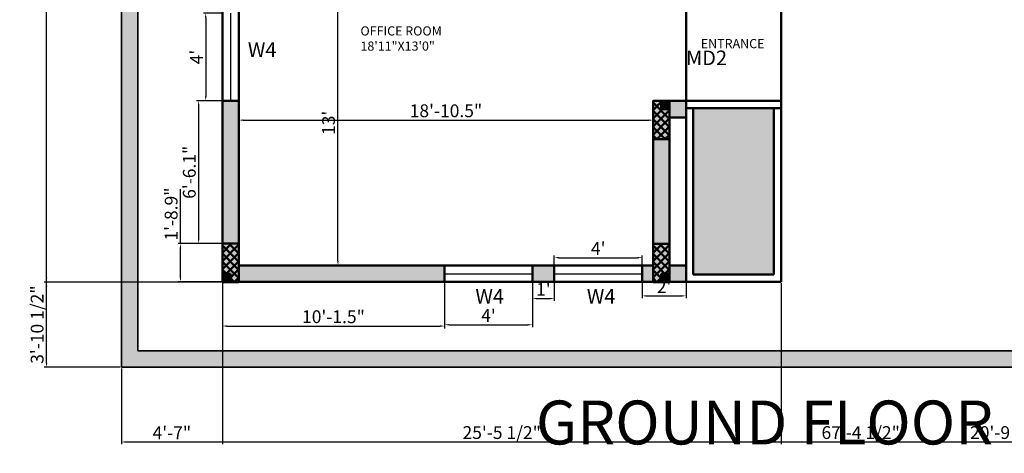
# Model space of a CAD drawing. Units: inches. Extents: x 1749 to 3550, y 1117 to 2383.
# Tile 6 of 15: x 1749 to 2287, y 1756 to 1993. Entities that reach past the tile are written whole.
import ezdxf

# ---------------------------------------------------------------- set-up
doc = ezdxf.new("R2010")
doc.units = ezdxf.units.IN
for name, color, linetype, lineweight in [('A-ANNO-DIMS', 2, 'Continuous', 18), ('A-ANNO-TEXT', 3, 'Continuous', 18), ('A-AREA-IDEN', 7, 'Continuous', 18), ('A-COLS', 10, 'Continuous', 50), ('A-GLAZ', 4, 'Continuous', 25), ('A-WALL', 7, 'Continuous', 50), ('A-WALL-PATT', 8, 'Continuous', 13), ('C-PROP', 8, 'Continuous', 35)]:
    doc.layers.add(name, color=color, linetype=linetype, lineweight=lineweight)
doc.styles.get("Standard").update_dxf_attribs({"font": 'arial.ttf'})
doc.dimstyles.new('ISO-25', dxfattribs={"dimtxt": 7, "dimasz": 2.5, "dimexe": 1.25, "dimexo": 0.625, "dimtad": 1, "dimdec": 1, "dimlunit": 3, "dimtxsty": 'Standard', "dimcen": 2.5, "dimadec": 0, "dimazin": 0, "dimtfac": 1, "dimtdec": 1, "dimtmove": 0, "dimatfit": 3, "dimfxl": 1, "dimarcsym": 0})

# ---------------------------------------------------------------- blocks, each defined once
blk = doc.blocks.new('*D6')
at = {"layer": 'A-ANNO-DIMS', "color": 0, "lineweight": -2, "transparency": 16777216}
for p, q in [((1923.39, 2014.66), (1924.02, 2014.66)), ((1922.77, 1861.16), (1922.77, 2012.16)), ((1923.39, 1858.66), (1924.02, 1858.66))]:
    blk.add_line(p, q, dxfattribs=at)
at = {"layer": 'A-ANNO-DIMS', "color": 0, "transparency": 16777216}
for points in [[(1922.35, 2012.16), (1923.18, 2012.16), (1922.77, 2014.66)], [(1922.35, 1861.16), (1923.18, 1861.16), (1922.77, 1858.66)]]:
    blk.add_solid(points, dxfattribs=at)
at = {"layer": 'Defpoints', "color": 0, "transparency": 16777216}
for p in [(1922.77, 2014.66), (1922.77, 2014.66), (1922.77, 1858.66)]:
    blk.add_point(p, dxfattribs=at)
at = {"layer": 'A-ANNO-DIMS', "color": 0, "transparency": 16777216, "insert": (1918.57, 1936.66), "char_height": 7, "attachment_point": 5, "rotation": 90}
blk.add_mtext("13'", dxfattribs=at)
blk = doc.blocks.new('*D7')
at = {"layer": 'A-ANNO-DIMS', "color": 0, "lineweight": -2, "transparency": 16777216}
for p, q in [((1868.6, 1948.04), (1868.6, 1936.91)), ((2095.1, 1948.04), (2095.1, 1936.91)), ((1871.1, 1938.16), (2092.6, 1938.16))]:
    blk.add_line(p, q, dxfattribs=at)
at = {"layer": 'A-ANNO-DIMS', "color": 0, "transparency": 16777216}
for points in [[(1871.1, 1938.58), (1871.1, 1937.74), (1868.6, 1938.16)], [(2092.6, 1938.58), (2092.6, 1937.74), (2095.1, 1938.16)]]:
    blk.add_solid(points, dxfattribs=at)
at = {"layer": 'Defpoints', "color": 0, "transparency": 16777216}
for p in [(1868.6, 1948.66), (2095.1, 1948.66), (2095.1, 1938.16)]:
    blk.add_point(p, dxfattribs=at)
at = {"layer": 'A-ANNO-DIMS', "color": 0, "transparency": 16777216, "insert": (1981.85, 1942.36), "char_height": 7, "attachment_point": 5}
blk.add_mtext('18\'-10.5"', dxfattribs=at)
blk = doc.blocks.new('*D88')
at = {"layer": 'A-ANNO-DIMS', "color": 0, "lineweight": -2, "ltscale": 0.5, "transparency": 16777216}
for p, q in [((1858.98, 1996.66), (1849.23, 1996.66)), ((1850.48, 1994.16), (1850.48, 1951.16)), ((1858.98, 1948.66), (1849.23, 1948.66))]:
    blk.add_line(p, q, dxfattribs=at)
at = {"layer": 'A-ANNO-DIMS', "color": 0, "ltscale": 0.5, "transparency": 16777216}
for points in [[(1850.06, 1994.16), (1850.89, 1994.16), (1850.48, 1996.66)], [(1850.06, 1951.16), (1850.89, 1951.16), (1850.48, 1948.66)]]:
    blk.add_solid(points, dxfattribs=at)
at = {"layer": 'Defpoints', "color": 0, "ltscale": 0.5, "transparency": 16777216}
for p in [(1859.6, 1996.66), (1850.48, 1948.66), (1859.6, 1948.66)]:
    blk.add_point(p, dxfattribs=at)
at = {"layer": 'A-ANNO-DIMS', "color": 0, "ltscale": 0.5, "transparency": 16777216, "insert": (1846.35, 1972.66), "char_height": 7, "attachment_point": 5, "rotation": 90}
blk.add_mtext("4'", dxfattribs=at)
blk = doc.blocks.new('*D89')
at = {"layer": 'A-ANNO-DIMS', "color": 0, "lineweight": -2, "ltscale": 0.5, "transparency": 16777216}
for p, q in [((1858.98, 1948.66), (1845.38, 1948.66)), ((1846.63, 1946.16), (1846.63, 1873.11)), ((1858.98, 1870.61), (1845.38, 1870.61))]:
    blk.add_line(p, q, dxfattribs=at)
at = {"layer": 'A-ANNO-DIMS', "color": 0, "ltscale": 0.5, "transparency": 16777216}
for points in [[(1846.21, 1946.16), (1847.04, 1946.16), (1846.63, 1948.66)], [(1846.21, 1873.11), (1847.04, 1873.11), (1846.63, 1870.61)]]:
    blk.add_solid(points, dxfattribs=at)
at = {"layer": 'Defpoints', "color": 0, "ltscale": 0.5, "transparency": 16777216}
for p in [(1859.6, 1948.66), (1846.63, 1870.61), (1859.6, 1870.61)]:
    blk.add_point(p, dxfattribs=at)
at = {"layer": 'A-ANNO-DIMS', "color": 0, "ltscale": 0.5, "transparency": 16777216, "insert": (1842.43, 1909.63), "char_height": 7, "attachment_point": 5, "rotation": 90}
blk.add_mtext('6\'-6.1"', dxfattribs=at)
blk = doc.blocks.new('*D90')
at = {"layer": 'A-ANNO-DIMS', "color": 0, "lineweight": -2, "ltscale": 0.5, "transparency": 16777216}
for p, q in [((1836.69, 1870.61), (1836.69, 1900.46)), ((1858.98, 1870.61), (1835.44, 1870.61)), ((1836.69, 1852.16), (1836.69, 1868.11)), ((1858.98, 1849.66), (1835.44, 1849.66))]:
    blk.add_line(p, q, dxfattribs=at)
at = {"layer": 'A-ANNO-DIMS', "color": 0, "ltscale": 0.5, "transparency": 16777216}
for points in [[(1836.28, 1868.11), (1837.11, 1868.11), (1836.69, 1870.61)], [(1836.28, 1852.16), (1837.11, 1852.16), (1836.69, 1849.66)]]:
    blk.add_solid(points, dxfattribs=at)
at = {"layer": 'Defpoints', "color": 0, "ltscale": 0.5, "transparency": 16777216}
for p in [(1836.69, 1870.61), (1859.6, 1870.61), (1859.6, 1849.66)]:
    blk.add_point(p, dxfattribs=at)
at = {"layer": 'A-ANNO-DIMS', "color": 0, "ltscale": 0.5, "transparency": 16777216, "insert": (1832.49, 1886.78), "char_height": 7, "attachment_point": 5, "rotation": 90}
blk.add_mtext('1\'-8.9"', dxfattribs=at)
blk = doc.blocks.new('*D91')
at = {"layer": 'A-ANNO-DIMS', "color": 0, "lineweight": -2, "ltscale": 0.5, "transparency": 16777216}
for p, q in [((1859.6, 1849.04), (1859.6, 1824.26)), ((1981.1, 1849.04), (1981.1, 1824.26)), ((1862.1, 1825.51), (1978.6, 1825.51))]:
    blk.add_line(p, q, dxfattribs=at)
at = {"layer": 'A-ANNO-DIMS', "color": 0, "ltscale": 0.5, "transparency": 16777216}
for points in [[(1862.1, 1825.93), (1862.1, 1825.1), (1859.6, 1825.51)], [(1978.6, 1825.93), (1978.6, 1825.1), (1981.1, 1825.51)]]:
    blk.add_solid(points, dxfattribs=at)
at = {"layer": 'Defpoints', "color": 0, "ltscale": 0.5, "transparency": 16777216}
for p in [(1859.6, 1849.66), (1981.1, 1849.66), (1981.1, 1825.51)]:
    blk.add_point(p, dxfattribs=at)
at = {"layer": 'A-ANNO-DIMS', "color": 0, "ltscale": 0.5, "transparency": 16777216, "insert": (1920.35, 1829.71), "char_height": 7, "attachment_point": 5}
blk.add_mtext('10\'-1.5"', dxfattribs=at)
blk = doc.blocks.new('*D92')
at = {"layer": 'A-ANNO-DIMS', "color": 0, "lineweight": -2, "ltscale": 0.5, "transparency": 16777216}
for p, q in [((1981.1, 1849.04), (1981.1, 1824.98)), ((2029.1, 1849.04), (2029.1, 1824.98)), ((1983.6, 1826.23), (2026.6, 1826.23))]:
    blk.add_line(p, q, dxfattribs=at)
at = {"layer": 'A-ANNO-DIMS', "color": 0, "ltscale": 0.5, "transparency": 16777216}
for points in [[(1983.6, 1826.64), (1983.6, 1825.81), (1981.1, 1826.23)], [(2026.6, 1826.64), (2026.6, 1825.81), (2029.1, 1826.23)]]:
    blk.add_solid(points, dxfattribs=at)
at = {"layer": 'Defpoints', "color": 0, "ltscale": 0.5, "transparency": 16777216}
for p in [(1981.1, 1849.66), (2029.1, 1849.66), (2029.1, 1826.23)]:
    blk.add_point(p, dxfattribs=at)
at = {"layer": 'A-ANNO-DIMS', "color": 0, "ltscale": 0.5, "transparency": 16777216, "insert": (2005.1, 1830.35), "char_height": 7, "attachment_point": 5}
blk.add_mtext("4'", dxfattribs=at)
blk = doc.blocks.new('*D93')
at = {"layer": 'A-ANNO-DIMS', "color": 0, "lineweight": -2, "ltscale": 0.5, "transparency": 16777216}
for p, q in [((2041.1, 1859.29), (2041.1, 1864.17)), ((2043.6, 1862.92), (2086.6, 1862.92)), ((2089.1, 1859.29), (2089.1, 1864.17))]:
    blk.add_line(p, q, dxfattribs=at)
at = {"layer": 'A-ANNO-DIMS', "color": 0, "ltscale": 0.5, "transparency": 16777216}
for points in [[(2043.6, 1863.34), (2043.6, 1862.51), (2041.1, 1862.92)], [(2086.6, 1863.34), (2086.6, 1862.51), (2089.1, 1862.92)]]:
    blk.add_solid(points, dxfattribs=at)
at = {"layer": 'Defpoints', "color": 0, "ltscale": 0.5, "transparency": 16777216}
for p in [(2089.1, 1862.92), (2041.1, 1858.66), (2089.1, 1858.66)]:
    blk.add_point(p, dxfattribs=at)
at = {"layer": 'A-ANNO-DIMS', "color": 0, "ltscale": 0.5, "transparency": 16777216, "insert": (2065.1, 1867.05), "char_height": 7, "attachment_point": 5}
blk.add_mtext("4'", dxfattribs=at)
blk = doc.blocks.new('*D94')
at = {"layer": 'A-ANNO-DIMS', "color": 0, "lineweight": -2, "ltscale": 0.5, "transparency": 16777216}
for p, q in [((2029.1, 1849.04), (2029.1, 1839.32)), ((2041.1, 1849.04), (2041.1, 1839.32)), ((2031.6, 1840.57), (2038.6, 1840.57))]:
    blk.add_line(p, q, dxfattribs=at)
at = {"layer": 'A-ANNO-DIMS', "color": 0, "ltscale": 0.5, "transparency": 16777216}
for points in [[(2031.6, 1840.98), (2031.6, 1840.15), (2029.1, 1840.57)], [(2038.6, 1840.98), (2038.6, 1840.15), (2041.1, 1840.57)]]:
    blk.add_solid(points, dxfattribs=at)
at = {"layer": 'Defpoints', "color": 0, "ltscale": 0.5, "transparency": 16777216}
for p in [(2029.1, 1849.66), (2041.1, 1849.66), (2041.1, 1840.57)]:
    blk.add_point(p, dxfattribs=at)
at = {"layer": 'A-ANNO-DIMS', "color": 0, "ltscale": 0.5, "transparency": 16777216, "insert": (2035.1, 1844.71), "char_height": 7, "attachment_point": 5}
blk.add_mtext("1'", dxfattribs=at)
blk = doc.blocks.new('*D95')
at = {"layer": 'A-ANNO-DIMS', "color": 0, "lineweight": -2, "ltscale": 0.5, "transparency": 16777216}
for p, q in [((2089.1, 1849.04), (2089.1, 1840.77)), ((2113.1, 1849.04), (2113.1, 1840.77)), ((2091.6, 1842.02), (2110.6, 1842.02))]:
    blk.add_line(p, q, dxfattribs=at)
at = {"layer": 'A-ANNO-DIMS', "color": 0, "ltscale": 0.5, "transparency": 16777216}
for points in [[(2091.6, 1842.43), (2091.6, 1841.6), (2089.1, 1842.02)], [(2110.6, 1842.43), (2110.6, 1841.6), (2113.1, 1842.02)]]:
    blk.add_solid(points, dxfattribs=at)
at = {"layer": 'Defpoints', "color": 0, "ltscale": 0.5, "transparency": 16777216}
for p in [(2089.1, 1849.66), (2113.1, 1849.66), (2113.1, 1842.02)]:
    blk.add_point(p, dxfattribs=at)
at = {"layer": 'A-ANNO-DIMS', "color": 0, "ltscale": 0.5, "transparency": 16777216, "insert": (2101.1, 1846.16), "char_height": 7, "attachment_point": 5}
blk.add_mtext("2'", dxfattribs=at)
blk = doc.blocks.new('*D157')
at = {"layer": 'A-ANNO-DIMS', "color": 0, "lineweight": -2, "ltscale": 0.5, "transparency": 16777216}
for p, q in [((1804.37, 1802.38), (1804.37, 1760.85)), ((2612.84, 1802.38), (2612.84, 1760.85)), ((1806.87, 1762.1), (2610.34, 1762.1))]:
    blk.add_line(p, q, dxfattribs=at)
at = {"layer": 'A-ANNO-DIMS', "color": 0, "ltscale": 0.5, "transparency": 16777216}
for points in [[(1806.87, 1762.52), (1806.87, 1761.69), (1804.37, 1762.1)], [(2610.34, 1762.52), (2610.34, 1761.69), (2612.84, 1762.1)]]:
    blk.add_solid(points, dxfattribs=at)
at = {"layer": 'Defpoints', "color": 0, "ltscale": 0.5, "transparency": 16777216}
for p in [(1804.37, 1803), (2612.84, 1803), (2612.84, 1762.1)]:
    blk.add_point(p, dxfattribs=at)
at = {"layer": 'A-ANNO-DIMS', "color": 0, "ltscale": 0.5, "transparency": 16777216, "insert": (2208.61, 1766.35), "char_height": 7, "attachment_point": 5}
blk.add_mtext('67\'-4 1/2"', dxfattribs=at)
blk = doc.blocks.new('*D158')
at = {"layer": 'A-ANNO-DIMS', "color": 0, "lineweight": -2, "ltscale": 0.5, "transparency": 16777216}
for p, q in [((1803.75, 2327.58), (1762.22, 2327.58)), ((1763.47, 1805.5), (1763.47, 2325.08)), ((1803.75, 1803), (1762.22, 1803))]:
    blk.add_line(p, q, dxfattribs=at)
at = {"layer": 'A-ANNO-DIMS', "color": 0, "ltscale": 0.5, "transparency": 16777216}
for points in [[(1763.05, 2325.08), (1763.89, 2325.08), (1763.47, 2327.58)], [(1763.05, 1805.5), (1763.89, 1805.5), (1763.47, 1803)]]:
    blk.add_solid(points, dxfattribs=at)
at = {"layer": 'Defpoints', "color": 0, "ltscale": 0.5, "transparency": 16777216}
for p in [(1763.47, 2327.58), (1804.37, 2327.58), (1804.37, 1803)]:
    blk.add_point(p, dxfattribs=at)
at = {"layer": 'A-ANNO-DIMS', "color": 0, "ltscale": 0.5, "transparency": 16777216, "insert": (1759.22, 2065.29), "char_height": 7, "attachment_point": 5, "rotation": 90}
blk.add_mtext('43\'-8 1/2"', dxfattribs=at)
blk = doc.blocks.new('*D160')
at = {"layer": 'A-ANNO-DIMS', "color": 0, "lineweight": -2, "ltscale": 0.5, "transparency": 16777216}
for p, q in [((1859.6, 1848.98), (1859.6, 1760.85)), ((1804.37, 1802.38), (1804.37, 1760.85)), ((1806.87, 1762.1), (1857.1, 1762.1))]:
    blk.add_line(p, q, dxfattribs=at)
at = {"layer": 'A-ANNO-DIMS', "color": 0, "ltscale": 0.5, "transparency": 16777216}
for points in [[(1806.87, 1762.52), (1806.87, 1761.69), (1804.37, 1762.1)], [(1857.1, 1762.52), (1857.1, 1761.69), (1859.6, 1762.1)]]:
    blk.add_solid(points, dxfattribs=at)
at = {"layer": 'Defpoints', "color": 0, "ltscale": 0.5, "transparency": 16777216}
for p in [(1859.6, 1849.61), (1804.37, 1803), (1859.6, 1762.1)]:
    blk.add_point(p, dxfattribs=at)
at = {"layer": 'A-ANNO-DIMS', "color": 0, "ltscale": 0.5, "transparency": 16777216, "insert": (1831.99, 1766.23), "char_height": 7, "attachment_point": 5}
blk.add_mtext('4\'-7"', dxfattribs=at)
blk = doc.blocks.new('*D161')
at = {"layer": 'A-ANNO-DIMS', "color": 0, "lineweight": -2, "ltscale": 0.5, "transparency": 16777216}
for p, q in [((1858.98, 1849.61), (1762.22, 1849.61)), ((1763.47, 1805.5), (1763.47, 1847.11)), ((1803.75, 1803), (1762.22, 1803))]:
    blk.add_line(p, q, dxfattribs=at)
at = {"layer": 'A-ANNO-DIMS', "color": 0, "ltscale": 0.5, "transparency": 16777216}
for points in [[(1763.05, 1847.11), (1763.89, 1847.11), (1763.47, 1849.61)], [(1763.05, 1805.5), (1763.89, 1805.5), (1763.47, 1803)]]:
    blk.add_solid(points, dxfattribs=at)
at = {"layer": 'Defpoints', "color": 0, "ltscale": 0.5, "transparency": 16777216}
for p in [(1763.47, 1849.61), (1859.6, 1849.61), (1804.37, 1803)]:
    blk.add_point(p, dxfattribs=at)
at = {"layer": 'A-ANNO-DIMS', "color": 0, "ltscale": 0.5, "transparency": 16777216, "insert": (1759.22, 1826.31), "char_height": 7, "attachment_point": 5, "rotation": 90}
blk.add_mtext('3\'-10 1/2"', dxfattribs=at)
blk = doc.blocks.new('*D162')
at = {"layer": 'A-ANNO-DIMS', "color": 0, "lineweight": -2, "ltscale": 0.5, "transparency": 16777216}
for p, q in [((1859.6, 1848.98), (1859.6, 1760.85)), ((2165.1, 1849.04), (2165.1, 1760.85)), ((1862.1, 1762.1), (2162.6, 1762.1))]:
    blk.add_line(p, q, dxfattribs=at)
at = {"layer": 'A-ANNO-DIMS', "color": 0, "ltscale": 0.5, "transparency": 16777216}
for points in [[(1862.1, 1762.52), (1862.1, 1761.69), (1859.6, 1762.1)], [(2162.6, 1762.52), (2162.6, 1761.69), (2165.1, 1762.1)]]:
    blk.add_solid(points, dxfattribs=at)
at = {"layer": 'Defpoints', "color": 0, "ltscale": 0.5, "transparency": 16777216}
for p in [(1859.6, 1849.61), (2165.1, 1849.66), (2165.1, 1762.1)]:
    blk.add_point(p, dxfattribs=at)
at = {"layer": 'A-ANNO-DIMS', "color": 0, "ltscale": 0.5, "transparency": 16777216, "insert": (2012.35, 1766.35), "char_height": 7, "attachment_point": 5}
blk.add_mtext('25\'-5 1/2"', dxfattribs=at)
blk = doc.blocks.new('*D163')
at = {"layer": 'A-ANNO-DIMS', "color": 0, "lineweight": -2, "ltscale": 0.5, "transparency": 16777216}
for p, q in [((1858.98, 2278.66), (1762.22, 2278.66)), ((1763.47, 1852.11), (1763.47, 2276.16)), ((1858.98, 1849.61), (1762.22, 1849.61))]:
    blk.add_line(p, q, dxfattribs=at)
at = {"layer": 'A-ANNO-DIMS', "color": 0, "ltscale": 0.5, "transparency": 16777216}
for points in [[(1763.05, 2276.16), (1763.89, 2276.16), (1763.47, 2278.66)], [(1763.05, 1852.11), (1763.89, 1852.11), (1763.47, 1849.61)]]:
    blk.add_solid(points, dxfattribs=at)
at = {"layer": 'Defpoints', "color": 0, "ltscale": 0.5, "transparency": 16777216}
for p in [(1763.47, 2278.66), (1859.6, 2278.66), (1859.6, 1849.61)]:
    blk.add_point(p, dxfattribs=at)
at = {"layer": 'A-ANNO-DIMS', "color": 0, "ltscale": 0.5, "transparency": 16777216, "insert": (1759.27, 2064.13), "char_height": 7, "attachment_point": 5, "rotation": 90}
blk.add_mtext('35\'-9"', dxfattribs=at)
blk = doc.blocks.new('*D167')
at = {"layer": 'A-ANNO-DIMS', "color": 0, "lineweight": -2, "ltscale": 0.5, "transparency": 16777216}
for p, q in [((2165.1, 1849.04), (2165.1, 1760.85)), ((2414.6, 1849.04), (2414.6, 1760.85)), ((2167.6, 1762.1), (2412.1, 1762.1))]:
    blk.add_line(p, q, dxfattribs=at)
at = {"layer": 'A-ANNO-DIMS', "color": 0, "ltscale": 0.5, "transparency": 16777216}
for points in [[(2167.6, 1762.52), (2167.6, 1761.69), (2165.1, 1762.1)], [(2412.1, 1762.52), (2412.1, 1761.69), (2414.6, 1762.1)]]:
    blk.add_solid(points, dxfattribs=at)
at = {"layer": 'Defpoints', "color": 0, "ltscale": 0.5, "transparency": 16777216}
for p in [(2165.1, 1849.66), (2414.6, 1849.66), (2414.6, 1762.1)]:
    blk.add_point(p, dxfattribs=at)
at = {"layer": 'A-ANNO-DIMS', "color": 0, "ltscale": 0.5, "transparency": 16777216, "insert": (2289.85, 1766.35), "char_height": 7, "attachment_point": 5}
blk.add_mtext('20\'-9 1/2"', dxfattribs=at)

msp = doc.modelspace()

# ---------------------------------------------------------------- hatches: boundary and pattern name
at = {"layer": 'A-COLS'}
h = msp.add_hatch(dxfattribs=at)
h.set_pattern_fill('ANSI37', color=256, angle=-90)
h.set_pattern_definition([(315, (323.5445, 4195.2253), (2.245064, 2.245064), []), (45, (323.5445, 4195.2253), (-2.245064, 2.245064), [])])
h.paths.add_polyline_path([(2104.1, 1948.66), (2095.1, 1948.66), (2095.1, 1927.66), (2104.1, 1927.66)])
h = msp.add_hatch(color=256, dxfattribs=at)
h.dxf.hatch_style = 1
h.paths.add_polyline_path([(2099.6, 1944.16), (2104.1, 1944.16), (2104.1, 1948.66), (2099.6, 1948.66)])
h = msp.add_hatch(dxfattribs=at)
h.set_pattern_fill('ANSI37', color=256, angle=-90)
h.set_pattern_definition([(315, (88.0445, 4117.1715), (2.245064, 2.245064), []), (45, (88.0445, 4117.1715), (-2.245064, 2.245064), [])])
h.paths.add_polyline_path([(1868.6, 1870.61), (1859.6, 1870.61), (1859.6, 1849.61), (1868.6, 1849.61)])
h = msp.add_hatch(dxfattribs=at)
h.set_pattern_fill('ANSI37', color=256, angle=-90)
h.set_pattern_definition([(315, (323.5445, 4117.105), (2.245064, 2.245064), []), (45, (323.5445, 4117.105), (-2.245064, 2.245064), [])])
h.paths.add_polyline_path([(2104.1, 1870.54), (2095.1, 1870.54), (2095.1, 1849.54), (2104.1, 1849.54)])
h = msp.add_hatch(color=256, dxfattribs=at)
h.dxf.hatch_style = 1
h.paths.add_polyline_path([(1859.6, 1849.66), (1864.1, 1849.66), (1864.1, 1854.16), (1859.6, 1854.16)])
h = msp.add_hatch(color=256, dxfattribs=at)
h.dxf.hatch_style = 1
h.paths.add_polyline_path([(2099.6, 1849.66), (2104.1, 1849.66), (2104.1, 1854.16), (2099.6, 1854.16)])
at = {"layer": 'A-WALL-PATT', "ltscale": 0.5}
h = msp.add_hatch(color=256, dxfattribs=at)
h.dxf.hatch_style = 1
h.paths.add_polyline_path([(2612.84, 2327.58), (1804.37, 2327.58), (1804.37, 1803), (2612.84, 1803), (2612.84, 2093.66), (2603.84, 2093.66), (2603.84, 1812), (1813.37, 1812), (1813.37, 2318.58), (2603.84, 2318.58), (2603.84, 2268.45), (2612.84, 2268.45)])
at = {"layer": 'A-WALL-PATT'}
h = msp.add_hatch(color=256, dxfattribs=at)
h.dxf.hatch_style = 1
h.paths.add_polyline_path([(2161.1, 2274.66), (2117.1, 2274.66), (2117.1, 2096.66), (2161.1, 2096.66)])
h.paths.add_polyline_path([(2161.1, 1944.66), (2117.1, 1944.66), (2117.1, 1853.66), (2161.1, 1853.66)])
h = msp.add_hatch(color=256, dxfattribs=at)
h.dxf.hatch_style = 1
h.paths.add_polyline_path([(1981.1, 1858.66), (1868.6, 1858.66), (1868.6, 1948.66), (1859.6, 1948.66), (1859.6, 1849.66), (1981.1, 1849.66)])
h = msp.add_hatch(color=256, dxfattribs=at)
h.dxf.hatch_style = 1
h.paths.add_polyline_path([(2104.1, 1939.66), (2113.1, 1939.66), (2113.1, 1948.66), (2095.1, 1948.66), (2095.1, 1858.66), (2089.1, 1858.66), (2089.1, 1849.66), (2113.1, 1849.66), (2113.1, 1858.66), (2104.1, 1858.66)])
h = msp.add_hatch(color=256, dxfattribs=at)
h.dxf.hatch_style = 1
h.paths.add_polyline_path([(2041.1, 1858.66), (2029.1, 1858.66), (2029.1, 1849.66), (2041.1, 1849.66)])

# ---------------------------------------------------------------- linework, layer by layer
at = {"layer": 'A-COLS'}
for p, q in [((2099.6, 1948.66), (2099.6, 1944.16)), ((2104.1, 1948.66), (2099.6, 1948.66)), ((2099.6, 1944.16), (2104.1, 1944.16)), ((2104.1, 1944.16), (2104.1, 1948.66)), ((1859.6, 1854.16), (1859.6, 1849.66)), ((1864.1, 1854.16), (1859.6, 1854.16)), ((1864.1, 1849.66), (1864.1, 1854.16)), ((2099.6, 1854.16), (2099.6, 1849.66)), ((2104.1, 1854.16), (2099.6, 1854.16)), ((2104.1, 1849.66), (2104.1, 1854.16)), ((1859.6, 1849.66), (1864.1, 1849.66)), ((2099.6, 1849.66), (2104.1, 1849.66))]:
    msp.add_line(p, q, dxfattribs=at)
for points in [[(2104.1, 1948.66), (2104.1, 1927.66), (2095.1, 1927.66), (2095.1, 1948.66)], [(1868.6, 1870.61), (1868.6, 1849.61), (1859.6, 1849.61), (1859.6, 1870.61)], [(2104.1, 1870.54), (2104.1, 1849.54), (2095.1, 1849.54), (2095.1, 1870.54)]]:
    msp.add_lwpolyline(points, close=True, dxfattribs=at)
at = {"layer": 'A-GLAZ'}
for p, q in [((1864.1, 1996.66), (1864.1, 1948.66)), ((1981.1, 1854.16), (2029.1, 1854.16)), ((2041.1, 1854.16), (2089.1, 1854.16))]:
    msp.add_line(p, q, dxfattribs=at)
at = {"layer": 'A-WALL'}
for p, q in [((2113.1, 2278.66), (2113.1, 1948.66)), ((2165.1, 2278.66), (2165.1, 1849.66)), ((1859.6, 2023.66), (1859.6, 1849.66)), ((1868.6, 2014.66), (1868.6, 1858.66)), ((1868.6, 1948.66), (1859.6, 1948.66)), ((2095.1, 1948.66), (2113.1, 1948.66)), ((2095.1, 1948.66), (2095.1, 1858.66)), ((2113.1, 1948.66), (2113.1, 1849.66)), ((2113.1, 1948.66), (2165.1, 1948.66)), ((2113.1, 1944.66), (2165.1, 1944.66)), ((2117.1, 1944.66), (2117.1, 1853.66)), ((2161.1, 1944.66), (2161.1, 1853.66)), ((2104.1, 1939.66), (2113.1, 1939.66)), ((2104.1, 1939.66), (2104.1, 1858.66)), ((1868.6, 1858.66), (2095.1, 1858.66)), ((1981.1, 1858.66), (1981.1, 1849.66)), ((2029.1, 1858.66), (2029.1, 1849.66)), ((2041.1, 1858.66), (2041.1, 1849.66)), ((2089.1, 1858.66), (2089.1, 1849.66)), ((2104.1, 1858.66), (2113.1, 1858.66)), ((2117.1, 1853.66), (2161.1, 1853.66)), ((1859.6, 1849.66), (2113.1, 1849.66)), ((2113.1, 1849.66), (2165.1, 1849.66))]:
    msp.add_line(p, q, dxfattribs=at)
at = {"layer": 'C-PROP', "ltscale": 0.5}
for p, q in [((1804.37, 1803), (1804.37, 2327.58)), ((1813.37, 1812), (1813.37, 2318.58)), ((2603.84, 1812), (1813.37, 1812)), ((2612.84, 1803), (1804.37, 1803))]:
    msp.add_line(p, q, dxfattribs=at)

# ---------------------------------------------------------------- texts
at = {"layer": 'A-ANNO-TEXT', "ltscale": 0.5}
for s, height, p in [('W4', 8, (1873.53, 1972.66)), ('MD2', 8, (2113.1, 1968.23)), ('W4', 8, (1997.94, 1837.81)), ('W4', 8, (2058.87, 1837.81)), ('GROUND FLOOR', 24, (2031.05, 1760.76))]:
    msp.add_text(s, height=height, dxfattribs=at).set_placement(p)
at = {"layer": 'A-AREA-IDEN', "ltscale": 0.5}
for s, p in [('OFFICE ROOM', (1935.1, 1984.45)), ('18\'11"X13\'0"', (1935.1, 1976.15)), ('ENTRANCE', (2121.18, 1977.51))]:
    msp.add_text(s, height=5, dxfattribs=at).set_placement(p)

# ---------------------------------------------------------------- dimensions: what is measured, and where the dimension line sits
at = {"layer": 'A-ANNO-DIMS', "ltscale": 0.5}
for base, p1, p2, override, picture, middle in [((1763.47, 2327.58), (1804.37, 1803), (1804.37, 2327.58), {"dimdec": 1, "dimlfac": 1, "dimrnd": 0, "dimzin": 1, "dimdsep": 46, "dimlunit": 4, "dimfrac": 2}, '*D158', (1759.22, 2065.29)), ((1763.4701, 2278.6615), (1859.6043, 1849.6077), (1859.6043, 2278.6615), {"dimdec": 1, "dimlfac": 1, "dimrnd": 0, "dimzin": 1, "dimdsep": 46, "dimlunit": 4, "dimfrac": 2}, '*D163', (1759.2687, 2064.1346)), ((1850.48, 1948.66), (1859.6, 1996.66), (1859.6, 1948.66), {"dimclrd": 0, "dimclre": 0, "dimclrt": 0}, '*D88', (1846.35, 1972.66)), ((1846.6269, 1870.6077), (1859.6043, 1948.6615), (1859.6043, 1870.6077), {"dimclrd": 0, "dimclre": 0, "dimclrt": 0}, '*D89', (1842.4279, 1909.6346)), ((1836.6924, 1870.6077), (1859.6043, 1849.6615), (1859.6043, 1870.6077), {"dimclrd": 0, "dimclre": 0, "dimclrt": 0}, '*D90', (1832.4934, 1886.7849)), ((1763.47, 1849.61), (1804.37, 1803), (1859.6, 1849.61), {"dimdec": 1, "dimlfac": 1, "dimrnd": 0, "dimzin": 1, "dimdsep": 46, "dimlunit": 4, "dimfrac": 2}, '*D161', (1759.22, 1826.31))]:
    dim = msp.add_linear_dim(base=base, p1=p1, p2=p2, angle=90, dimstyle='ISO-25', override=override, dxfattribs=at)
    dim.commit()
    dim.dimension.update_dxf_attribs({"geometry": picture, "text_midpoint": middle})
at = {"layer": 'A-ANNO-DIMS'}
dim = msp.add_linear_dim(base=(1922.77, 2014.66), p1=(1922.77, 1858.66), p2=(1922.77, 2014.66), angle=90, dimstyle='ISO-25', override={"dimclrd": 0, "dimclre": 0, "dimclrt": 0}, dxfattribs=at)
dim.commit()
dim.dimension.update_dxf_attribs({"geometry": '*D6', "text_midpoint": (1918.57, 1936.66)})
dim = msp.add_linear_dim(base=(2095.1, 1938.16), p1=(1868.6, 1948.66), p2=(2095.1, 1948.66), dimstyle='ISO-25', override={"dimclrd": 0, "dimclre": 0, "dimclrt": 0}, dxfattribs=at)
dim.commit()
dim.dimension.update_dxf_attribs({"geometry": '*D7', "text_midpoint": (1981.85, 1942.36)})
at = {"layer": 'A-ANNO-DIMS', "ltscale": 0.5}
for base, p1, p2, override, picture, middle in [((2089.1, 1862.92), (2041.1, 1858.66), (2089.1, 1858.66), {"dimclrd": 0, "dimclre": 0, "dimclrt": 0}, '*D93', (2065.1, 1867.05)), ((1859.6, 1762.1), (1804.37, 1803), (1859.6, 1849.61), {"dimdec": 1, "dimlfac": 1, "dimrnd": 0, "dimzin": 1, "dimdsep": 46, "dimlunit": 4, "dimfrac": 2}, '*D160', (1831.99, 1766.23)), ((1981.1, 1825.51), (1859.6, 1849.66), (1981.1, 1849.66), {"dimclrd": 0, "dimclre": 0, "dimclrt": 0}, '*D91', (1920.35, 1829.71)), ((2165.1, 1762.1), (1859.6, 1849.61), (2165.1, 1849.66), {"dimdec": 1, "dimlfac": 1, "dimrnd": 0, "dimzin": 1, "dimdsep": 46, "dimlunit": 4, "dimfrac": 2}, '*D162', (2012.35, 1766.35)), ((2029.1, 1826.23), (1981.1, 1849.66), (2029.1, 1849.66), {"dimclrd": 0, "dimclre": 0, "dimclrt": 0}, '*D92', (2005.1, 1830.35)), ((2041.1, 1840.57), (2029.1, 1849.66), (2041.1, 1849.66), {"dimclrd": 0, "dimclre": 0, "dimclrt": 0}, '*D94', (2035.1, 1844.71)), ((2113.1, 1842.02), (2089.1, 1849.66), (2113.1, 1849.66), {"dimclrd": 0, "dimclre": 0, "dimclrt": 0}, '*D95', (2101.1, 1846.16)), ((2414.6, 1762.1), (2165.1, 1849.66), (2414.6, 1849.66), {"dimdec": 1, "dimlfac": 1, "dimrnd": 0, "dimzin": 1, "dimdsep": 46, "dimlunit": 4, "dimfrac": 2}, '*D167', (2289.85, 1766.35)), ((2612.84, 1762.1), (1804.37, 1803), (2612.84, 1803), {"dimdec": 1, "dimlfac": 1, "dimrnd": 0, "dimzin": 1, "dimdsep": 46, "dimlunit": 4, "dimfrac": 2}, '*D157', (2208.61, 1766.35))]:
    dim = msp.add_linear_dim(base=base, p1=p1, p2=p2, dimstyle='ISO-25', override=override, dxfattribs=at)
    dim.commit()
    dim.dimension.update_dxf_attribs({"geometry": picture, "text_midpoint": middle})

doc.saveas('drawing.dxf')
